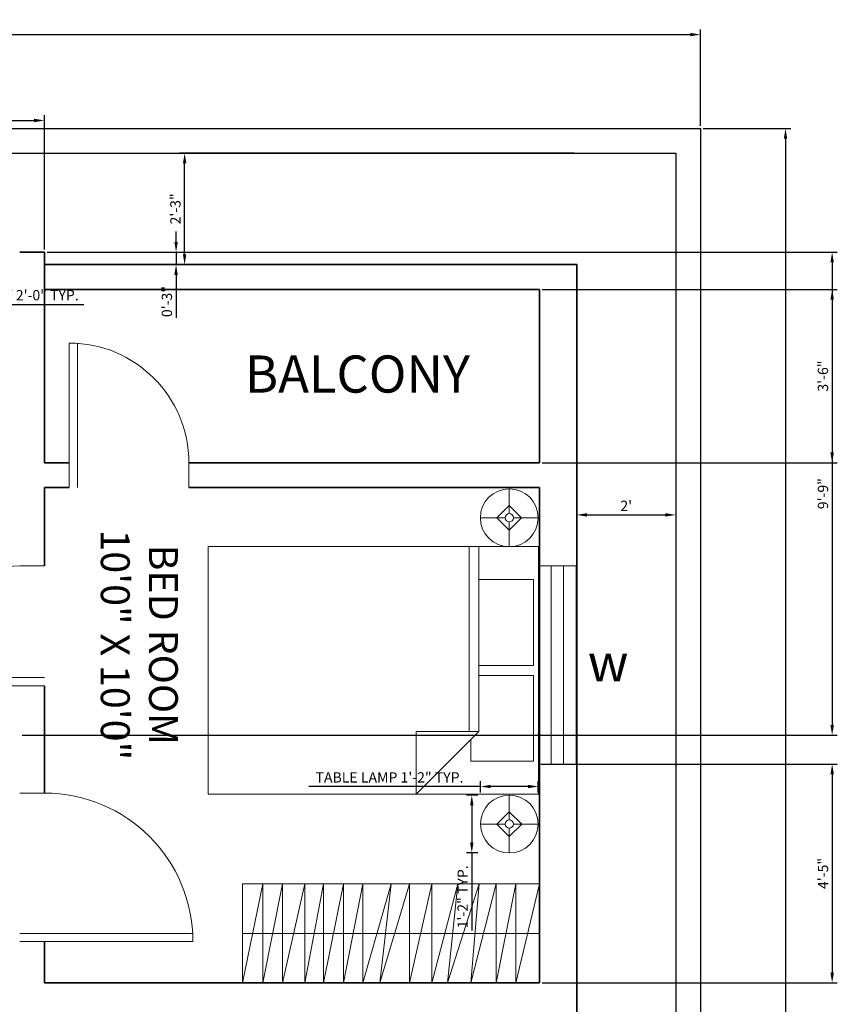
# Model space of a CAD drawing. Units: inches. Extents: x 1879 to 2382, y 1769 to 2461.
# Tile 5 of 5: x 2183 to 2381, y 2190 to 2429. Entities that reach past the tile are written whole.
import ezdxf

# ---------------------------------------------------------------- set-up
doc = ezdxf.new("R2010")
doc.units = ezdxf.units.IN
for name, color, linetype, lineweight in [('A-ANNO-DIMS', 2, 'Continuous', 18), ('A-ANNO-TEXT', 3, 'Continuous', 18), ('A-AREA-IDEN', 7, 'Continuous', 18), ('A-DOOR', 3, 'Continuous', 18), ('A-FLOR-CASE', 8, 'Continuous', 18), ('A-FURN', 9, 'Continuous', 18), ('A-GLAZ', 4, 'Continuous', 18), ('A-WALL', 7, 'Continuous', 35), ('C-PROP', 1, 'Continuous', 25)]:
    doc.layers.add(name, color=color, linetype=linetype, lineweight=lineweight)
doc.styles.get("Standard").update_dxf_attribs({"font": 'arial.ttf'})
doc.dimstyles.new('ISO-25', dxfattribs={"dimtxt": 2.5, "dimasz": 2.5, "dimexe": 1.25, "dimexo": 0.625, "dimtad": 1, "dimlunit": 4, "dimtxsty": 'Standard', "dimcen": 2.5, "dimadec": 0, "dimazin": 0, "dimtfac": 1, "dimtmove": 0, "dimatfit": 3, "dimfxl": 1, "dimarcsym": 0})

# ---------------------------------------------------------------- blocks, each defined once
blk = doc.blocks.new('*D1')
at = {"layer": 'A-ANNO-DIMS', "color": 0, "lineweight": -2, "transparency": 16777216}
for p, q in [((1916.34, 2402.81), (1916.34, 2426.16)), ((2348.34, 2402.81), (2348.34, 2426.16)), ((1918.84, 2424.91), (2345.84, 2424.91))]:
    blk.add_line(p, q, dxfattribs=at)
at = {"layer": 'A-ANNO-DIMS', "color": 0, "transparency": 16777216}
for points in [[(1918.84, 2425.32), (1918.84, 2424.49), (1916.34, 2424.91)], [(2345.84, 2425.32), (2345.84, 2424.49), (2348.34, 2424.91)]]:
    blk.add_solid(points, dxfattribs=at)
at = {"layer": 'Defpoints', "color": 0, "transparency": 16777216}
for p in [(2348.34, 2424.91), (1916.34, 2402.18), (2348.34, 2402.18)]:
    blk.add_point(p, dxfattribs=at)
at = {"layer": 'A-ANNO-DIMS', "color": 0, "transparency": 16777216, "insert": (2132.34, 2426.81), "char_height": 2.5, "attachment_point": 5}
blk.add_mtext("36'", dxfattribs=at)
blk = doc.blocks.new('*D2')
at = {"layer": 'A-ANNO-DIMS', "color": 0, "lineweight": -2, "transparency": 16777216}
for p, q in [((2348.97, 2402.18), (2370.19, 2402.18)), ((2368.94, 2399.68), (2368.94, 1804.68)), ((2348.97, 1802.18), (2370.19, 1802.18))]:
    blk.add_line(p, q, dxfattribs=at)
at = {"layer": 'A-ANNO-DIMS', "color": 0, "transparency": 16777216}
for points in [[(2368.53, 2399.68), (2369.36, 2399.68), (2368.94, 2402.18)], [(2368.53, 1804.68), (2369.36, 1804.68), (2368.94, 1802.18)]]:
    blk.add_solid(points, dxfattribs=at)
at = {"layer": 'Defpoints', "color": 0, "transparency": 16777216}
for p in [(2348.34, 2402.18), (2348.34, 1802.18), (2368.94, 1802.18)]:
    blk.add_point(p, dxfattribs=at)
at = {"layer": 'A-ANNO-DIMS', "color": 0, "transparency": 16777216, "insert": (2367.04, 2102.18), "char_height": 2.5, "attachment_point": 5, "rotation": 90}
blk.add_mtext("50'", dxfattribs=at)
blk = doc.blocks.new('Bed - Queen')
for p, q in [((0, -80.00003), (0, 0)), ((0, 0), (59.99999, 0)), ((59.99999, 0), (59.99999, -80.00003)), ((7.99999, -1.2), (28.79998, -1.2)), ((7.99999, -14.4), (7.99999, -1.2)), ((28.79998, -1.2), (28.79998, -14.4)), ((31.19999, -1.2), (51.99999, -1.2)), ((31.19999, -14.4), (31.19999, -1.2)), ((51.99999, -1.2), (51.99999, -16.4)), ((0, -14.4), (44.8, -14.4)), ((59.99999, -29.6), (44.8, -14.4)), ((44.8, -14.4), (44.8, -29.6)), ((51.99999, -16.4), (46.79936, -16.4)), ((44.8, -16.8), (0, -16.8)), ((44.8, -29.6), (59.99999, -29.6)), ((59.99999, -80.00003), (0, -80.00003))]:
    blk.add_line(p, q)
blk = doc.blocks.new('Lamp - Table')
for p, q in [((0, 7), (0, 1)), ((0, 3), (-3, 0)), ((3, 0), (0, 3)), ((-1, 0), (-7, 0)), ((-3, 0), (0, -3)), ((0, -3), (3, 0)), ((1, 0), (7, 0)), ((0, -1), (0, -7))]:
    blk.add_line(p, q)
for radius in [7, 1]:
    blk.add_circle((0, 0), radius)
blk = doc.blocks.new('*D15')
at = {"layer": 'A-ANNO-DIMS', "color": 0, "lineweight": -2, "transparency": 16777216}
for p, q in [((2317.72, 2396.18), (2222.06, 2396.18)), ((2223.31, 2371.68), (2223.31, 2393.68)), ((2317.72, 2369.18), (2222.06, 2369.18))]:
    blk.add_line(p, q, dxfattribs=at)
at = {"layer": 'A-ANNO-DIMS', "color": 0, "transparency": 16777216}
for points in [[(2222.9, 2393.68), (2223.73, 2393.68), (2223.31, 2396.18)], [(2222.9, 2371.68), (2223.73, 2371.68), (2223.31, 2369.18)]]:
    blk.add_solid(points, dxfattribs=at)
at = {"layer": 'Defpoints', "color": 0, "transparency": 16777216}
for p in [(2223.31, 2396.18), (2318.34, 2396.18), (2318.34, 2369.18)]:
    blk.add_point(p, dxfattribs=at)
at = {"layer": 'A-ANNO-DIMS', "color": 0, "transparency": 16777216, "insert": (2221.41, 2382.68), "char_height": 2.5, "attachment_point": 5, "rotation": 90}
blk.add_mtext('2\'-3"', dxfattribs=at)
blk = doc.blocks.new('*D16')
at = {"layer": 'A-ANNO-DIMS', "color": 0, "lineweight": -2, "transparency": 16777216}
for p, q in [((2318.34, 2368.56), (2318.34, 2307.3)), ((2342.34, 2368.56), (2342.34, 2307.3)), ((2320.84, 2308.55), (2339.84, 2308.55))]:
    blk.add_line(p, q, dxfattribs=at)
at = {"layer": 'A-ANNO-DIMS', "color": 0, "transparency": 16777216}
for points in [[(2320.84, 2308.97), (2320.84, 2308.14), (2318.34, 2308.55)], [(2339.84, 2308.97), (2339.84, 2308.14), (2342.34, 2308.55)]]:
    blk.add_solid(points, dxfattribs=at)
at = {"layer": 'Defpoints', "color": 0, "transparency": 16777216}
for p in [(2318.34, 2369.18), (2342.34, 2369.18), (2342.34, 2308.55)]:
    blk.add_point(p, dxfattribs=at)
at = {"layer": 'A-ANNO-DIMS', "color": 0, "transparency": 16777216, "insert": (2330.34, 2310.43), "char_height": 2.5, "width": 2.3431, "attachment_point": 5}
blk.add_mtext("2'", dxfattribs=at)
blk = doc.blocks.new('WN-48x9')
for p, q in [((0, 48), (0, 0)), ((9, 48), (0, 48)), ((3, 48), (3, 0)), ((6, 0), (6, 48)), ((9, 0), (9, 48)), ((0, 0), (9, 0))]:
    blk.add_line(p, q)
blk = doc.blocks.new('DR-SWING-29')
for p, q in [((27, 6), (27, 35)), ((29, 6), (29, 35)), ((0, 0), (0, 6)), ((27, 6), (27, 0)), ((29, 6), (29, 0))]:
    blk.add_line(p, q)
blk.add_arc((29, 6), 29, 90, 180)
blk = doc.blocks.new('DR-SWING-36')
for p, q in [((42, 36), (36, 36)), ((36, 2), (0, 2)), ((36, 0), (0, 0)), ((36, 2), (42, 2)), ((36, 0), (42, 0))]:
    blk.add_line(p, q)
blk.add_arc((36, 0), 36, 90, 180)
blk = doc.blocks.new('WARDROBE-HANGERS-72')
for p, q in [((0, 0), (4.89, 24)), ((4.89, 24), (4.89, 0)), ((4.89, 0), (9.67, 24)), ((9.67, 24), (9.67, 0)), ((9.67, 0), (15.08, 24)), ((15.08, 24), (15.08, 0)), ((15.08, 0), (19.6, 24)), ((19.6, 24), (19.6, 0)), ((19.6, 0), (24.51, 24)), ((24.51, 24), (24.51, 0)), ((24.51, 0), (29.16, 24)), ((29.16, 24), (29.16, 0)), ((29.16, 0), (36, 24)), ((36, 24), (33.31, 0)), ((33.31, 0), (40.47, 24)), ((40.47, 24), (40.47, 0)), ((40.47, 0), (45.88, 24)), ((45.88, 24), (45.88, 0)), ((45.88, 0), (52.17, 24)), ((52.17, 24), (49.65, 0)), ((49.65, 0), (57.32, 24)), ((57.32, 24), (55.31, 0)), ((55.31, 0), (61.47, 24)), ((61.47, 24), (61.47, 0)), ((61.47, 0), (66.25, 24)), ((66.25, 24), (66.25, 0)), ((66.25, 0), (72, 24))]:
    blk.add_line(p, q)
blk = doc.blocks.new('*D35')
at = {"layer": 'A-ANNO-DIMS', "color": 0, "lineweight": -2, "transparency": 16777216}
for p, q in [((2145.46, 2362.53), (2145.46, 2358.3)), ((2169.46, 2362.53), (2169.46, 2358.3)), ((2147.96, 2359.55), (2166.96, 2359.55)), ((2169.46, 2359.55), (2198.87, 2359.55))]:
    blk.add_line(p, q, dxfattribs=at)
at = {"layer": 'A-ANNO-DIMS', "color": 0, "transparency": 16777216}
for points in [[(2147.96, 2359.97), (2147.96, 2359.14), (2145.46, 2359.55)], [(2166.96, 2359.97), (2166.96, 2359.14), (2169.46, 2359.55)]]:
    blk.add_solid(points, dxfattribs=at)
at = {"layer": 'Defpoints', "color": 0, "transparency": 16777216}
for p in [(2145.46, 2363.15), (2169.46, 2363.15), (2169.46, 2359.55)]:
    blk.add_point(p, dxfattribs=at)
at = {"layer": 'A-ANNO-DIMS', "color": 0, "transparency": 16777216, "insert": (2185.41, 2361.45), "char_height": 2.5, "attachment_point": 5}
blk.add_mtext('VENT 2\'-0" TYP.', dxfattribs=at)
blk = doc.blocks.new('*D41')
at = {"layer": 'A-ANNO-DIMS', "color": 0, "lineweight": -2, "transparency": 16777216}
for p, q in [((2295.01, 2242.76), (2253.44, 2242.76)), ((2295.01, 2241.28), (2295.01, 2244.01)), ((2306.51, 2242.76), (2297.51, 2242.76)), ((2309.01, 2241.28), (2309.01, 2244.01))]:
    blk.add_line(p, q, dxfattribs=at)
at = {"layer": 'A-ANNO-DIMS', "color": 0, "transparency": 16777216}
for points in [[(2297.51, 2243.17), (2297.51, 2242.34), (2295.01, 2242.76)], [(2306.51, 2243.17), (2306.51, 2242.34), (2309.01, 2242.76)]]:
    blk.add_solid(points, dxfattribs=at)
at = {"layer": 'Defpoints', "color": 0, "transparency": 16777216}
for p in [(2295.01, 2242.76), (2295.01, 2240.66), (2309.01, 2240.66)]:
    blk.add_point(p, dxfattribs=at)
at = {"layer": 'A-ANNO-DIMS', "color": 0, "transparency": 16777216, "insert": (2272.97, 2244.64), "char_height": 2.5, "attachment_point": 5}
blk.add_mtext('TABLE LAMP 1\'-2" TYP.', dxfattribs=at)
blk = doc.blocks.new('*D42')
at = {"layer": 'A-ANNO-DIMS', "color": 0, "lineweight": -2, "transparency": 16777216}
for p, q in [((2294.38, 2240.66), (2291.66, 2240.66)), ((2292.91, 2238.16), (2292.91, 2229.16)), ((2294.38, 2226.66), (2291.66, 2226.66)), ((2292.91, 2226.66), (2292.91, 2207.9))]:
    blk.add_line(p, q, dxfattribs=at)
at = {"layer": 'A-ANNO-DIMS', "color": 0, "transparency": 16777216}
for points in [[(2292.49, 2238.16), (2293.32, 2238.16), (2292.91, 2240.66)], [(2292.49, 2229.16), (2293.32, 2229.16), (2292.91, 2226.66)]]:
    blk.add_solid(points, dxfattribs=at)
at = {"layer": 'Defpoints', "color": 0, "transparency": 16777216}
for p in [(2295.01, 2240.66), (2292.91, 2226.66), (2295.01, 2226.66)]:
    blk.add_point(p, dxfattribs=at)
at = {"layer": 'A-ANNO-DIMS', "color": 0, "transparency": 16777216, "insert": (2291.02, 2216.03), "char_height": 2.5, "attachment_point": 5, "rotation": 90}
blk.add_mtext('1\'-2" TYP.', dxfattribs=at)
blk = doc.blocks.new('*D58')
at = {"layer": 'A-ANNO-DIMS', "color": 0, "lineweight": -2, "transparency": 16777216}
for p, q in [((2309.97, 2363.18), (2381.49, 2363.18)), ((2380.24, 2360.68), (2380.24, 2323.68)), ((2309.97, 2321.18), (2381.49, 2321.18))]:
    blk.add_line(p, q, dxfattribs=at)
at = {"layer": 'A-ANNO-DIMS', "color": 0, "transparency": 16777216}
for points in [[(2379.82, 2360.68), (2380.66, 2360.68), (2380.24, 2363.18)], [(2379.82, 2323.68), (2380.66, 2323.68), (2380.24, 2321.18)]]:
    blk.add_solid(points, dxfattribs=at)
at = {"layer": 'Defpoints', "color": 0, "transparency": 16777216}
for p in [(2309.34, 2363.18), (2309.34, 2321.18), (2380.24, 2321.18)]:
    blk.add_point(p, dxfattribs=at)
at = {"layer": 'A-ANNO-DIMS', "color": 0, "transparency": 16777216, "insert": (2378.34, 2342.18), "char_height": 2.5, "attachment_point": 5, "rotation": 90}
blk.add_mtext('3\'-6"', dxfattribs=at)
blk = doc.blocks.new('*D74')
at = {"layer": 'A-ANNO-DIMS', "color": 0, "lineweight": -2, "transparency": 16777216}
for p, q in [((2309.8, 2248.19), (2381.49, 2248.19)), ((2380.24, 2245.69), (2380.24, 2197.68)), ((2309.97, 2195.18), (2381.49, 2195.18))]:
    blk.add_line(p, q, dxfattribs=at)
at = {"layer": 'A-ANNO-DIMS', "color": 0, "transparency": 16777216}
for points in [[(2379.82, 2245.69), (2380.66, 2245.69), (2380.24, 2248.19)], [(2379.82, 2197.68), (2380.66, 2197.68), (2380.24, 2195.18)]]:
    blk.add_solid(points, dxfattribs=at)
at = {"layer": 'Defpoints', "color": 0, "transparency": 16777216}
for p in [(2309.17, 2248.19), (2309.34, 2195.18), (2380.24, 2195.18)]:
    blk.add_point(p, dxfattribs=at)
at = {"layer": 'A-ANNO-DIMS', "color": 0, "transparency": 16777216, "insert": (2378.35, 2221.69), "char_height": 2.5, "attachment_point": 5, "rotation": 90}
blk.add_mtext('4\'-5"', dxfattribs=at)
blk = doc.blocks.new('*D78')
at = {"layer": 'A-ANNO-DIMS', "color": 0, "lineweight": -2, "transparency": 16777216}
for p, q in [((2085.34, 2372.81), (2085.33, 2405.33)), ((2189.34, 2372.83), (2189.33, 2405.35)), ((2087.84, 2404.08), (2186.84, 2404.1))]:
    blk.add_line(p, q, dxfattribs=at)
at = {"layer": 'A-ANNO-DIMS', "color": 0, "transparency": 16777216}
for points in [[(2087.84, 2404.5), (2087.84, 2403.66), (2085.34, 2404.08)], [(2186.84, 2404.52), (2186.84, 2403.68), (2189.34, 2404.1)]]:
    blk.add_solid(points, dxfattribs=at)
at = {"layer": 'Defpoints', "color": 0, "transparency": 16777216}
for p in [(2189.34, 2404.1), (2085.34, 2372.18), (2189.34, 2372.2)]:
    blk.add_point(p, dxfattribs=at)
at = {"layer": 'A-ANNO-DIMS', "color": 0, "transparency": 16777216, "insert": (2137.33, 2405.99), "char_height": 2.5, "attachment_point": 5, "rotation": 0.0111}
blk.add_mtext('8\'-8"', dxfattribs=at)
blk = doc.blocks.new('*D79')
at = {"layer": 'A-ANNO-DIMS', "color": 0, "lineweight": -2, "transparency": 16777216}
for p, q in [((2189.97, 2372.2), (2381.49, 2372.2)), ((2380.24, 2369.7), (2380.24, 2257.68)), ((2183.97, 2255.18), (2381.49, 2255.18))]:
    blk.add_line(p, q, dxfattribs=at)
at = {"layer": 'A-ANNO-DIMS', "color": 0, "transparency": 16777216}
for points in [[(2379.82, 2369.7), (2380.66, 2369.7), (2380.24, 2372.2)], [(2379.82, 2257.68), (2380.66, 2257.68), (2380.24, 2255.18)]]:
    blk.add_solid(points, dxfattribs=at)
at = {"layer": 'Defpoints', "color": 0, "transparency": 16777216}
for p in [(2189.34, 2372.2), (2183.34, 2255.18), (2380.24, 2255.18)]:
    blk.add_point(p, dxfattribs=at)
at = {"layer": 'A-ANNO-DIMS', "color": 0, "transparency": 16777216, "insert": (2378.34, 2313.69), "char_height": 2.5, "attachment_point": 5, "rotation": 90}
blk.add_mtext('9\'-9"', dxfattribs=at)
blk = doc.blocks.new('*D80')
at = {"layer": 'A-ANNO-DIMS', "color": 0, "lineweight": -2, "transparency": 16777216}
for p, q in [((2221.24, 2374.7), (2221.24, 2377.2)), ((2189.97, 2372.2), (2222.49, 2372.2)), ((2221.24, 2372.2), (2221.24, 2369.18)), ((2189.97, 2369.18), (2222.49, 2369.18)), ((2221.24, 2366.68), (2221.24, 2356.28))]:
    blk.add_line(p, q, dxfattribs=at)
at = {"layer": 'A-ANNO-DIMS', "color": 0, "transparency": 16777216}
for points in [[(2220.82, 2374.7), (2221.66, 2374.7), (2221.24, 2372.2)], [(2220.82, 2366.68), (2221.66, 2366.68), (2221.24, 2369.18)]]:
    blk.add_solid(points, dxfattribs=at)
at = {"layer": 'Defpoints', "color": 0, "transparency": 16777216}
for p in [(2189.34, 2372.2), (2189.34, 2369.18), (2221.24, 2369.18)]:
    blk.add_point(p, dxfattribs=at)
at = {"layer": 'A-ANNO-DIMS', "color": 0, "transparency": 16777216, "insert": (2219.34, 2360.23), "char_height": 2.5, "attachment_point": 5, "rotation": 90}
blk.add_mtext('0\'-3"', dxfattribs=at)

msp = doc.modelspace()

# ---------------------------------------------------------------- linework, layer by layer
at = {"layer": 'A-FLOR-CASE'}
for p, q in [((2309.341, 2219.18), (2237.341, 2219.18)), ((2237.341, 2219.18), (2237.341, 2195.18)), ((2309.341, 2195.18), (2309.341, 2219.18)), ((2237.341, 2207.18), (2309.341, 2207.18))]:
    msp.add_line(p, q, dxfattribs=at)
at = {"layer": 'A-WALL'}
for p, q in [((2189.341, 2372.201), (2183.341, 2372.18)), ((2189.341, 2363.18), (2189.341, 2372.201)), ((2189.341, 2369.18), (2309.341, 2369.18)), ((2309.341, 2369.18), (2318.341, 2369.18)), ((2318.341, 2369.18), (2318.341, 1808.18)), ((2189.341, 2363.18), (2189.341, 2321.18)), ((2189.341, 2363.18), (2309.341, 2363.18)), ((2309.341, 2363.18), (2309.341, 2321.18)), ((2189.341, 2321.18), (2195.341, 2321.18)), ((2189.341, 2321.18), (2195.341, 2321.18)), ((2224.341, 2321.18), (2309.341, 2321.18)), ((2189.341, 2315.18), (2195.341, 2315.18)), ((2189.341, 2315.18), (2189.341, 2296.18)), ((2224.341, 2315.18), (2309.341, 2315.18)), ((2309.341, 2315.18), (2309.341, 2195.18)), ((2189.341, 2267.18), (2189.341, 2241.18)), ((2189.341, 2195.18), (2189.341, 2205.18)), ((2189.341, 2205.18), (2189.341, 2195.18)), ((2189.341, 2195.18), (2309.341, 2195.18))]:
    msp.add_line(p, q, dxfattribs=at)
at = {"layer": 'C-PROP'}
for p, q in [((1916.341, 2402.18), (2348.341, 2402.18)), ((2348.341, 2402.18), (2348.341, 1802.18)), ((1922.341, 2396.18), (2342.341, 2396.18)), ((2342.341, 2396.18), (2342.341, 1808.18))]:
    msp.add_line(p, q, dxfattribs=at)

# ---------------------------------------------------------------- block references
at = {"layer": 'A-DOOR', "extrusion": (0, 0, -1), "zscale": -1}
for name, p in [('DR-SWING-29', (-2224.341, 2315.18)), ('DR-SWING-36', (-2225.341, 2205.18))]:
    msp.add_blockref(name, p, dxfattribs=at)
at = {"layer": 'A-DOOR', "extrusion": (0, 0, -1), "zscale": -1, "rotation": 269.9999999999997}
msp.add_blockref('DR-SWING-29', (-2189.341, 2296.18), dxfattribs=at)
at = {"layer": 'A-FLOR-CASE'}
msp.add_blockref('WARDROBE-HANGERS-72', (2237.341, 2195.18), dxfattribs=at)
at = {"layer": 'A-FURN'}
for name, p, rotation in [('Lamp - Table', (2301.993, 2307.859), 180), ('Bed - Queen', (2309.04, 2300.866), 270), ('Lamp - Table', (2302.005, 2233.657), 180)]:
    msp.add_blockref(name, p, dxfattribs=dict(at, rotation=rotation))
at = {"layer": 'A-GLAZ'}
msp.add_blockref('WN-48x9', (2309.171, 2248.194), dxfattribs=at)

# ---------------------------------------------------------------- texts
at = {"layer": 'A-ANNO-TEXT', "insert": (2269.834, 2277.236), "char_height": 9, "attachment_point": 1}
msp.add_mtext_dynamic_manual_height_columns('\\pxqc;w', width=112.22887, gutter_width=12.5, heights=[0], dxfattribs=at)
at = {"layer": 'A-AREA-IDEN', "insert": (2237.92, 2347.173), "char_height": 9, "attachment_point": 1}
msp.add_mtext_dynamic_manual_height_columns('BALCONY', width=86.90732, gutter_width=12.5, heights=[0], dxfattribs=at)
at = {"layer": 'A-AREA-IDEN', "insert": (2221.675, 2323.151), "char_height": 7, "attachment_point": 1, "rotation": 270}
msp.add_mtext_dynamic_manual_height_columns('\\pxqc;BED ROOM\\P10\'0" X 10\'0"', width=92.15185, gutter_width=12.5, heights=[0], dxfattribs=at)

# ---------------------------------------------------------------- dimensions: what is measured, and where the dimension line sits
at = {"layer": 'A-ANNO-DIMS'}
for base, p1, p2, picture, middle in [((2348.341, 2424.907), (1916.341, 2402.18), (2348.341, 2402.18), '*D1', (2132.341, 2426.81)), ((2342.341, 2308.553), (2318.341, 2369.18), (2342.341, 2369.18), '*D16', (2330.341, 2310.433))]:
    dim = msp.add_linear_dim(base=base, p1=p1, p2=p2, dimstyle='ISO-25', override={"dimclrd": 0, "dimclre": 0, "dimclrt": 0}, dxfattribs=at)
    dim.commit()
    dim.dimension.update_dxf_attribs({"geometry": picture, "text_midpoint": middle})
for base, p1, p2, angle, override, picture, middle in [((2189.335, 2404.101), (2085.341, 2372.181), (2189.341, 2372.201), 0.01114, {"dimdec": 1, "dimlfac": 1, "dimrnd": 0, "dimzin": 1, "dimdsep": 46, "dimlunit": 4, "dimfrac": 2}, '*D78', (2137.335, 2405.992)), ((2368.943, 1802.18), (2348.341, 2402.18), (2348.341, 1802.18), 90, {"dimclrd": 0, "dimclre": 0, "dimclrt": 0}, '*D2', (2367.042, 2102.18)), ((2223.313, 2396.18), (2318.341, 2369.18), (2318.341, 2396.18), 90, {"dimclrd": 0, "dimclre": 0, "dimclrt": 0}, '*D15', (2221.411, 2382.68)), ((2221.241, 2369.18), (2189.341, 2372.201), (2189.341, 2369.18), 270, {"dimdec": 1, "dimlfac": 1, "dimrnd": 0, "dimzin": 1, "dimdsep": 46, "dimlunit": 4, "dimfrac": 2}, '*D80', (2219.339, 2360.233)), ((2380.241, 2255.18), (2189.341, 2372.201), (2183.341, 2255.18), 90, {"dimdec": 1, "dimlfac": 1, "dimrnd": 0, "dimzin": 1, "dimdsep": 46, "dimlunit": 4, "dimfrac": 2}, '*D79', (2378.34, 2313.691)), ((2380.241, 2321.18), (2309.341, 2363.18), (2309.341, 2321.18), 90, {"dimdec": 1, "dimlfac": 1, "dimrnd": 0, "dimzin": 1, "dimdsep": 46, "dimlunit": 4, "dimfrac": 2}, '*D58', (2378.339, 2342.18)), ((2380.241, 2195.18), (2309.171, 2248.194), (2309.341, 2195.18), 90, {"dimdec": 1, "dimlfac": 1, "dimrnd": 0, "dimzin": 1, "dimdsep": 46, "dimlunit": 4, "dimfrac": 2}, '*D74', (2378.345, 2221.687))]:
    dim = msp.add_linear_dim(base=base, p1=p1, p2=p2, angle=angle, dimstyle='ISO-25', override=override, dxfattribs=at)
    dim.commit()
    dim.dimension.update_dxf_attribs({"geometry": picture, "text_midpoint": middle})
dim = msp.add_linear_dim(base=(2169.463, 2359.553), p1=(2145.463, 2363.153), p2=(2169.463, 2363.153), text='VENT <> TYP.', dimstyle='ISO-25', override={"dimdec": 1, "dimlfac": 1, "dimrnd": 0, "dimzin": 1, "dimdsep": 46, "dimlunit": 4, "dimfrac": 2}, dxfattribs=at)
dim.commit()
dim.dimension.update_dxf_attribs({"geometry": '*D35', "text_midpoint": (2185.415, 2361.454)})
for base, p1, p2, angle, text, picture, middle in [((2295.005, 2242.757), (2309.005, 2240.657), (2295.005, 2240.657), 180, 'TABLE LAMP <> TYP.', '*D41', (2272.972, 2244.638)), ((2292.905, 2226.657), (2295.005, 2240.657), (2295.005, 2226.657), 270, '<> TYP.', '*D42', (2291.024, 2216.03))]:
    dim = msp.add_linear_dim(base=base, p1=p1, p2=p2, angle=angle, text=text, dimstyle='ISO-25', override={"dimdec": 1, "dimlfac": 1, "dimrnd": 0, "dimzin": 1, "dimdsep": 46, "dimlunit": 4, "dimfrac": 2}, dxfattribs=at)
    dim.commit()
    dim.dimension.update_dxf_attribs({"geometry": picture, "text_midpoint": middle})

doc.saveas('drawing.dxf')
